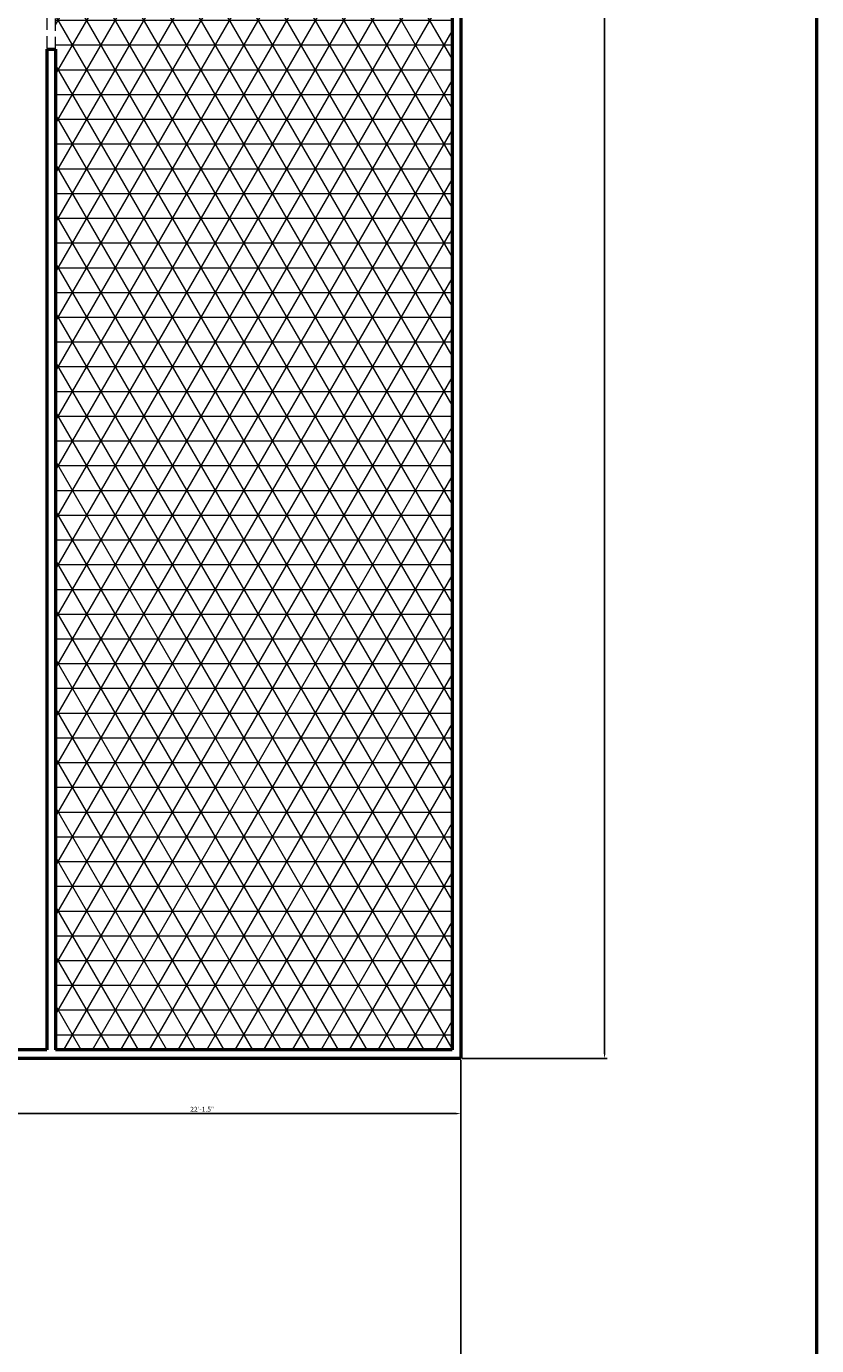
# Model space of a CAD drawing. Units: millimetres. Extents: x 1945 to 2943, y 628 to 2340.
# Tile 3 of 5: x 2538 to 2943, y 977 to 1654. Entities that reach past the tile are written whole.
import ezdxf

# ---------------------------------------------------------------- set-up
doc = ezdxf.new("R2010")
doc.units = ezdxf.units.MM
doc.linetypes.add('DASHED', pattern=[19.05, 12.7, -6.35])
for name, color, linetype, lineweight in [('A-ANNO-DIMS', 2, 'Continuous', 18), ('A-FLOR-PATT', 8, 'Continuous', 13), ('A-WALL', 7, 'Continuous', 50), ('A-WALL-OPNG', 8, 'DASHED', 18)]:
    doc.layers.add(name, color=color, linetype=linetype, lineweight=lineweight)
doc.styles.get("Standard").update_dxf_attribs({"font": 'arial.ttf'})
doc.dimstyles.new('ISO-25', dxfattribs={"dimtxt": 2.5, "dimasz": 2.5, "dimexe": 1.25, "dimexo": 0.625, "dimtad": 1, "dimlunit": 3, "dimtxsty": 'Standard', "dimcen": 2.5, "dimadec": 0, "dimazin": 0, "dimtfac": 1, "dimtmove": 0, "dimatfit": 3, "dimfxl": 1, "dimarcsym": 0})

# ---------------------------------------------------------------- blocks, each defined once
blk = doc.blocks.new('*D12')
at = {"layer": 'A-ANNO-DIMS', "color": 0, "lineweight": -2, "transparency": 16777216}
for p, q in [((2761.22, 2252.62), (2835.55, 2252.62)), ((2834.3, 2250.12), (2834.3, 1126.62)), ((2761.22, 1124.12), (2835.55, 1124.12))]:
    blk.add_line(p, q, dxfattribs=at)
at = {"layer": 'A-ANNO-DIMS', "color": 0, "transparency": 16777216}
for points in [[(2833.88, 2250.12), (2834.71, 2250.12), (2834.3, 2252.62)], [(2833.88, 1126.62), (2834.71, 1126.62), (2834.3, 1124.12)]]:
    blk.add_solid(points, dxfattribs=at)
at = {"layer": 'Defpoints', "color": 0, "transparency": 16777216}
for p in [(2760.6, 2252.62), (2760.6, 1124.12), (2834.3, 1124.12)]:
    blk.add_point(p, dxfattribs=at)
at = {"layer": 'A-ANNO-DIMS', "color": 0, "transparency": 16777216, "insert": (2832.4, 1688.37), "char_height": 2.5, "attachment_point": 5, "rotation": 90}
blk.add_mtext('94\'-0.5"', dxfattribs=at)
blk = doc.blocks.new('*D16')
at = {"layer": 'A-ANNO-DIMS', "color": 0, "lineweight": -2, "ltscale": 0.5, "transparency": 16777216}
for p, q in [((2760.6, 1123.5), (2760.6, 1094.64)), ((2495.1, 1107.96), (2495.1, 1094.64)), ((2497.6, 1095.89), (2758.1, 1095.89))]:
    blk.add_line(p, q, dxfattribs=at)
at = {"layer": 'A-ANNO-DIMS', "color": 0, "ltscale": 0.5, "transparency": 16777216}
for points in [[(2497.6, 1096.31), (2497.6, 1095.47), (2495.1, 1095.89)], [(2758.1, 1096.31), (2758.1, 1095.47), (2760.6, 1095.89)]]:
    blk.add_solid(points, dxfattribs=at)
at = {"layer": 'Defpoints', "color": 0, "ltscale": 0.5, "transparency": 16777216}
for p in [(2760.6, 1124.12), (2495.1, 1108.59), (2760.6, 1095.89)]:
    blk.add_point(p, dxfattribs=at)
at = {"layer": 'A-ANNO-DIMS', "color": 0, "ltscale": 0.5, "transparency": 16777216, "insert": (2627.85, 1097.79), "char_height": 2.5, "attachment_point": 5}
blk.add_mtext('22\'-1.5"', dxfattribs=at)
blk = doc.blocks.new('*D24')
at = {"layer": 'A-ANNO-DIMS', "color": 0, "lineweight": -2, "transparency": 16777216}
for p, q in [((2760.6, 1123.5), (2760.6, 857.56)), ((2029.02, 989.8), (2029.02, 857.56)), ((2031.52, 858.81), (2758.1, 858.81))]:
    blk.add_line(p, q, dxfattribs=at)
at = {"layer": 'A-ANNO-DIMS', "color": 0, "transparency": 16777216}
for points in [[(2031.52, 859.23), (2031.52, 858.39), (2029.02, 858.81)], [(2758.1, 859.23), (2758.1, 858.39), (2760.6, 858.81)]]:
    blk.add_solid(points, dxfattribs=at)
at = {"layer": 'Defpoints', "color": 0, "transparency": 16777216}
for p in [(2760.6, 1124.12), (2029.02, 990.43), (2760.6, 858.81)]:
    blk.add_point(p, dxfattribs=at)
at = {"layer": 'A-ANNO-DIMS', "color": 0, "transparency": 16777216, "insert": (2394.81, 860.73), "char_height": 2.5, "attachment_point": 5}
blk.add_mtext('60\'-11 1/2"', dxfattribs=at)

msp = doc.modelspace()

# ---------------------------------------------------------------- hatches: boundary and pattern name
at = {"layer": 'A-FLOR-PATT'}
h = msp.add_hatch(dxfattribs=at)
h.set_pattern_fill('NET3', color=256, scale=4)
h.set_pattern_definition([(0, (1094.862, 577.549), (0, 12.7), []), (60, (1094.862, 577.549), (-10.99852, 6.35), []), (120, (1094.862, 577.549), (-10.99852, -6.35), [])])
h.paths.add_polyline_path([(2756.097, 2086.621), (2751.597, 2086.621), (2751.597, 2094.839), (2552.597, 2094.839), (2552.597, 2091.121), (2582.597, 2091.121), (2582.597, 2089.809), (2582.569, 2089.809, -0.4014527), (2552.597, 2061.121), (2552.597, 1128.621), (2756.097, 1128.621)])

# ---------------------------------------------------------------- linework, layer by layer
at = {"layer": 'A-WALL'}
for p, q in [((2760.597, 2252.621), (2760.597, 1124.121)), ((2756.097, 2086.621), (2756.097, 1128.621)), ((2548.097, 1642.145), (2548.097, 1128.621)), ((2552.597, 1642.145), (2552.597, 1128.621)), ((2548.097, 1128.621), (2495.097, 1128.621)), ((2760.597, 1124.121), (2495.097, 1124.121)), ((2756.097, 1128.621), (2552.597, 1128.621))]:
    msp.add_line(p, q, dxfattribs=at)
at = {"layer": 'A-WALL', "ltscale": 0.5}
msp.add_line((2548.097, 1642.145), (2552.597, 1642.145), dxfattribs=at)
msp.add_lwpolyline([(1944.667, 2340.145), (2943.065, 2340.145), (2943.065, 839.363), (1944.667, 839.363)], close=True, dxfattribs=at)
at = {"layer": 'A-WALL-OPNG', "ltscale": 0.5}
for p, q in [((2548.097, 1791.761), (2548.097, 1642.145)), ((2552.597, 1642.145), (2552.597, 1791.761)), ((2548.097, 1642.145), (2552.597, 1642.145))]:
    msp.add_line(p, q, dxfattribs=at)

# ---------------------------------------------------------------- dimensions: what is measured, and where the dimension line sits
at = {"layer": 'A-ANNO-DIMS'}
dim = msp.add_linear_dim(base=(2834.297, 1124.121), p1=(2760.597, 2252.621), p2=(2760.597, 1124.121), angle=90, dimstyle='ISO-25', override={"dimclrd": 0, "dimclre": 0, "dimclrt": 0}, dxfattribs=at)
dim.commit()
dim.dimension.update_dxf_attribs({"geometry": '*D12', "text_midpoint": (2832.395, 1688.371)})
dim = msp.add_linear_dim(base=(2760.597, 858.809), p1=(2029.018, 990.428), p2=(2760.597, 1124.121), dimstyle='ISO-25', override={"dimdec": 1, "dimlfac": 1, "dimrnd": 0, "dimzin": 1, "dimdsep": 46, "dimlunit": 4, "dimfrac": 2}, dxfattribs=at)
dim.commit()
dim.dimension.update_dxf_attribs({"geometry": '*D24', "text_midpoint": (2394.808, 860.727)})
at = {"layer": 'A-ANNO-DIMS', "ltscale": 0.5}
dim = msp.add_linear_dim(base=(2760.597, 1095.89), p1=(2495.097, 1108.589), p2=(2760.597, 1124.121), dimstyle='ISO-25', override={"dimclrd": 0, "dimclre": 0, "dimclrt": 0}, dxfattribs=at)
dim.commit()
dim.dimension.update_dxf_attribs({"geometry": '*D16', "text_midpoint": (2627.847, 1097.791)})

doc.saveas('drawing.dxf')
